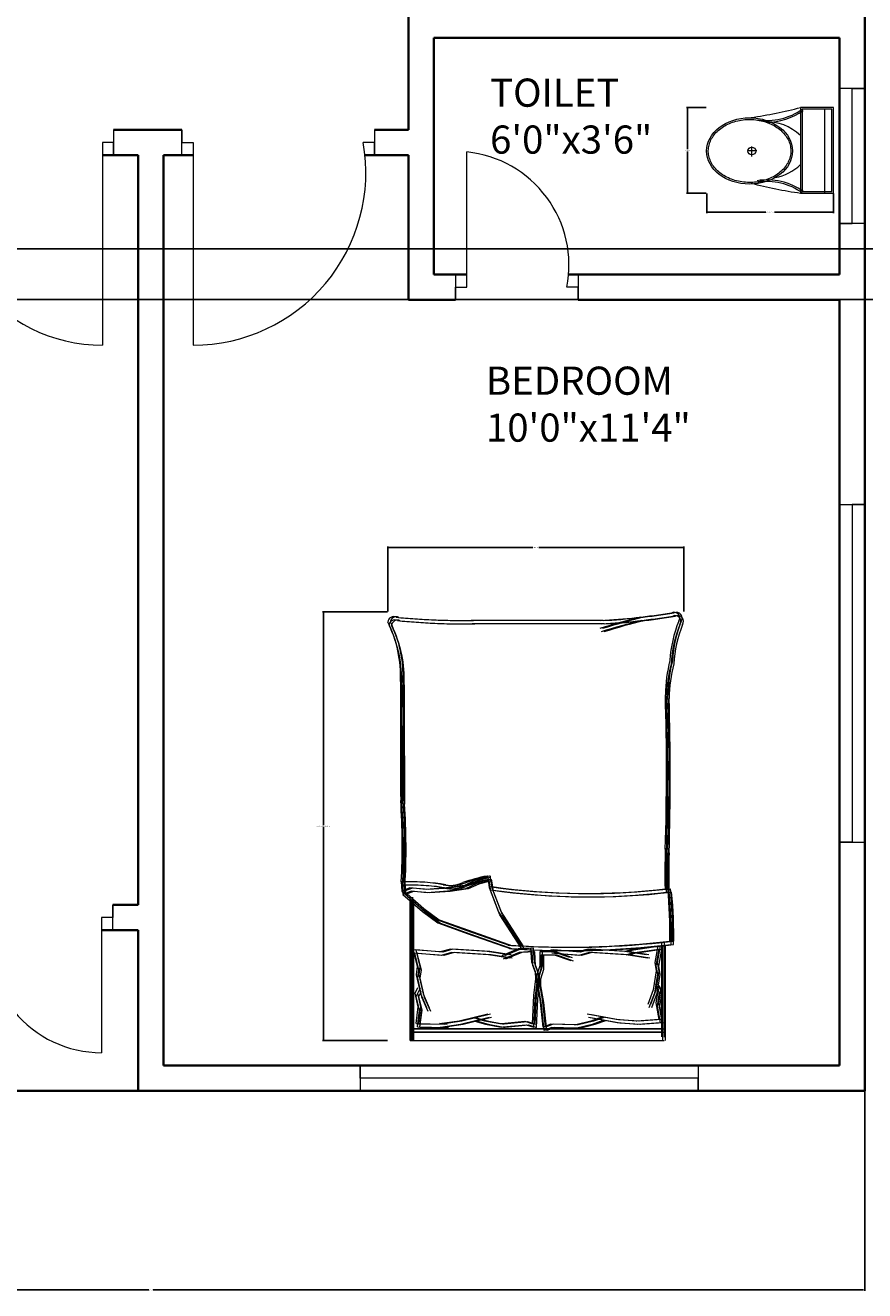
# Model space of a CAD drawing. Units: inches. Extents: x 2234 to 3001, y 1541 to 2386.
# Tile 3 of 12: x 2739 to 2888, y 1667 to 1891. Entities that reach past the tile are written whole.
import ezdxf

# ---------------------------------------------------------------- set-up
doc = ezdxf.new("R2010")
doc.units = ezdxf.units.IN
for name, color, linetype, lineweight in [('A-ANNO-DIMS', 2, 'Continuous', 18), ('A-AREA-IDEN', 7, 'Continuous', 18), ('A-DOOR', 3, 'Continuous', 18), ('A-FLOR-FIXT', 9, 'Continuous', 18), ('A-FURN', 9, 'Continuous', 13), ('A-GLAZ', 4, 'Continuous', 18), ('A-WALL', 7, 'Continuous', 35)]:
    doc.layers.add(name, color=color, linetype=linetype, lineweight=lineweight)
doc.styles.get("Standard").update_dxf_attribs({"font": 'arial.ttf'})
doc.dimstyles.get("Standard").update_dxf_attribs({"dimtxt": 0.18, "dimasz": 0.18, "dimexe": 0.18, "dimexo": 0.0625, "dimgap": 0.09, "dimtad": 0, "dimtih": 1, "dimtoh": 1, "dimdec": 4, "dimzin": 0, "dimdsep": 46, "dimtxsty": 'Standard', "dimcen": 0.09, "dimadec": 0, "dimazin": 0, "dimtfac": 1, "dimtdec": 4, "dimtofl": 0, "dimtmove": 0, "dimatfit": 3, "dimfxl": 1, "dimtolj": 1, "dimtzin": 0, "dimarcsym": 0})

# ---------------------------------------------------------------- blocks, each defined once
blk = doc.blocks.new('A$C31115884')
for p, q in [((283.1, 497.7), (223.4, 497.7)), ((257.5, 466.4), (257.5, 523.2)), ((0, 200), (0, 0)), ((520, 200), (0, 200)), ((10, 190), (10, 10)), ((510, 190), (10, 190)), ((510, 10), (510, 190)), ((520, 0), (520, 200)), ((510, 54.5), (0, 54.5)), ((10, 10), (510, 10)), ((0, 0), (520, 0))]:
    blk.add_line(p, q)
blk.add_circle((255.6, 496.4), 23.6)
for centre, radius, start, end in [((2777.7, -204.6), 2807, 165.4549, 171.71327), ((-294.5, 403.3), 364.7, 324.20913, 9.34987), ((-294.5, 403.3), 374.7, 324.20913, 9.34987), ((805.8, 403.3), 364.7, 170.65013, 215.79087), ((3237, 905), 2807, 188.28673, 194.5451), ((139.5, 406.2), 293.5, 315.84364, 2.65635), ((805.8, 403.3), 374.7, 179.20365, 215.79087), ((383.6, 406.2), 293.5, 190.27735, 224.15636)]:
    blk.add_arc(centre, radius, start, end)
blk.add_ellipse((256.2, 509.9), major_axis=(0, -260.7), ratio=0.772727)
blk.add_open_spline([(256.2, 259.2), (263.1, 259.2), (270, 259.7), (287.8, 262.3), (298.7, 265.1), (319.9, 273.1), (330.2, 278.4), (350.1, 291.1), (359.7, 298.7), (377.7, 315.9), (386.2, 325.5), (401.7, 346.6), (408.8, 358.1), (421.3, 382.5), (426.8, 395.5), (435.9, 422.4), (439.5, 436.4), (444.8, 465.1), (446.5, 479.7), (447.9, 509.2), (447.6, 524), (445, 553.3), (442.7, 567.8), (436.3, 596), (432.1, 609.7), (421.9, 636), (416, 648.6), (402.5, 672.1), (395, 683), (378.6, 703), (369.8, 712.1), (351.1, 728), (341.3, 734.8), (320.9, 746.2), (310.4, 750.7), (288.9, 757.3), (278, 759.4), (256, 761), (245, 760.6), (223.1, 757.2), (212.3, 754.3), (191.1, 746.1), (180.8, 740.7), (160.9, 727.8), (151.4, 720.1), (133.5, 702.7), (125.1, 693), (109.6, 671.7), (102.6, 660.2), (90.2, 635.7), (84.9, 622.7), (76, 595.6), (72.4, 581.6), (67.2, 552.9), (65.6, 538.2), (64.4, 508.8), (64.8, 494), (67.5, 464.7), (69.9, 450.2), (76.6, 422), (80.8, 408.3), (91.1, 382.2), (97.2, 369.7), (110.8, 346.3), (118.4, 335.4), (134.8, 315.6), (143.7, 306.7), (162.4, 290.9), (172.3, 284.2), (192.8, 273), (203.3, 268.6), (224.8, 262.2), (235.8, 260.2), (249.9, 259.3), (253, 259.2), (256.2, 259.2)], degree=3, knots=[0, 0, 0, 0, 0.110105, 0.110105, 0.285049, 0.285049, 0.459994, 0.459994, 0.634938, 0.634938, 0.809882, 0.809882, 0.984827, 0.984827, 1.159771, 1.159771, 1.334715, 1.334715, 1.50966, 1.50966, 1.684604, 1.684604, 1.859549, 1.859549, 2.034493, 2.034493, 2.209437, 2.209437, 2.384382, 2.384382, 2.559326, 2.559326, 2.73427, 2.73427, 2.909215, 2.909215, 3.084159, 3.084159, 3.259103, 3.259103, 3.434048, 3.434048, 3.608992, 3.608992, 3.783936, 3.783936, 3.958881, 3.958881, 4.133825, 4.133825, 4.30877, 4.30877, 4.483714, 4.483714, 4.658658, 4.658658, 4.833603, 4.833603, 5.008547, 5.008547, 5.183491, 5.183491, 5.358436, 5.358436, 5.53338, 5.53338, 5.708324, 5.708324, 5.883269, 5.883269, 6.058213, 6.058213, 6.233158, 6.233158, 6.283185, 6.283185, 6.283185, 6.283185])
blk = doc.blocks.new('WIN-60-A')
for p, q in [((0, 60), (4.5, 60)), ((4.5, 60), (2.25, 60)), ((2.25, 60), (2.25, 0)), ((2.25, 0), (0, 0)), ((0, 0), (4.5, 0))]:
    blk.add_line(p, q)
blk = doc.blocks.new('WIN-24-A')
for p, q in [((0, 24), (4.5, 24)), ((4.5, 24), (2.25, 24)), ((2.25, 24), (2.25, 0)), ((2.25, 0), (0, 0)), ((0, 0), (4.5, 0))]:
    blk.add_line(p, q)
blk = doc.blocks.new('BED-DOUBLE-B')
for p, q in [((37.77, 74.61), (14.78, 74.61)), ((37.77, 74.61), (14.78, 74.61)), ((38.22, 74.59), (15.24, 74.59)), ((38.22, 74.59), (15.24, 74.59)), ((37.98, 74.02), (15, 74.02)), ((37.98, 74.02), (15, 74.02)), ((38.44, 73.99), (15.45, 73.99)), ((38.44, 73.99), (15.46, 73.99)), ((2.39, 28.15), (2.47, 26.53, 3.61)), ((2.39, 28.15), (2.47, 26.53, 3.61)), ((3.9, 27.1), (2.47, 26.53)), ((3.9, 27.1), (2.47, 26.53)), ((2.61, 27.56), (2.68, 25.93, 3.61)), ((2.61, 27.56), (2.68, 25.93, 3.61)), ((2.85, 28.13), (2.92, 26.5, 3.61)), ((2.85, 28.13), (2.93, 26.5, 3.61)), ((4.36, 27.08), (2.92, 26.5)), ((4.36, 27.08), (2.93, 26.5)), ((3.06, 27.54), (3.14, 25.91, 3.61)), ((3.06, 27.54), (3.14, 25.91, 3.61)), ((6.79, 26.81), (3.9, 27.1)), ((6.8, 26.81), (3.9, 27.1)), ((7.25, 26.79), (4.36, 27.08)), ((7.25, 26.79), (4.36, 27.08)), ((10.41, 27.1), (6.79, 26.81)), ((10.41, 27.1), (6.8, 26.81)), ((10.87, 27.08), (7.25, 26.79)), ((10.87, 27.08), (7.25, 26.79)), ((13.59, 27.54), (10.41, 27.1)), ((13.59, 27.54), (10.41, 27.1)), ((14.05, 27.52), (10.87, 27.08)), ((14.05, 27.52), (10.87, 27.08)), ((15.47, 28.4), (13.59, 27.54)), ((15.47, 28.4), (13.59, 27.54)), ((15.68, 27.81), (13.8, 26.94)), ((15.69, 27.81), (13.81, 26.94)), ((15.93, 28.38), (14.05, 27.52)), ((15.93, 28.38), (14.05, 27.52)), ((16.14, 27.79), (14.26, 26.92)), ((16.14, 27.79), (14.26, 26.92)), ((17.79, 28.98), (15.47, 28.4)), ((17.79, 28.98), (15.47, 28.4)), ((18, 28.38), (15.68, 27.81)), ((18, 28.38), (15.69, 27.81)), ((18.24, 28.96), (15.93, 28.38)), ((18.24, 28.96), (15.93, 28.38)), ((18.46, 28.36), (16.14, 27.79)), ((18.46, 28.36), (16.14, 27.79)), ((18.07, 27.1), (17.79, 28.98)), ((18.07, 27.1), (17.79, 28.98)), ((18.29, 26.51), (18, 28.38)), ((18.29, 26.51), (18, 28.38)), ((19.67, 22.91), (18.07, 27.1)), ((19.67, 22.91), (18.07, 27.1)), ((18.53, 27.08), (18.24, 28.96)), ((18.53, 27.08), (18.24, 28.96)), ((18.75, 26.49), (18.46, 28.36)), ((18.75, 26.49), (18.46, 28.36)), ((20.12, 22.89), (18.53, 27.08)), ((20.12, 22.89), (18.53, 27.08)), ((2.47, 26.53), (5.93, 23.49)), ((2.47, 26.53), (5.93, 23.49)), ((4.12, 26.51), (2.68, 25.93)), ((4.12, 26.51), (2.68, 25.93)), ((2.68, 25.93), (6.14, 22.89)), ((2.68, 25.93), (6.14, 22.89)), ((2.92, 26.5), (6.38, 23.47)), ((2.93, 26.5), (6.39, 23.47)), ((4.57, 26.49), (3.14, 25.91)), ((4.57, 26.49), (3.14, 25.91)), ((3.14, 25.91), (6.6, 22.87)), ((3.14, 25.91), (6.6, 22.87)), ((3.96, 0.62), (3.96, 25.46)), ((3.96, 0.62), (3.96, 25.46)), ((7.01, 26.22), (4.12, 26.51)), ((7.01, 26.22), (4.12, 26.51)), ((4.18, 0.02), (4.18, 24.87)), ((4.18, 0.02), (4.18, 24.87)), ((4.42, 0.6), (4.42, 25.44)), ((4.42, 0.6), (4.42, 25.44)), ((7.47, 26.2), (4.57, 26.49)), ((7.47, 26.2), (4.57, 26.49)), ((4.63, 0), (4.63, 24.85)), ((4.63, 0), (4.63, 24.85)), ((10.62, 26.51), (7.01, 26.22)), ((10.62, 26.51), (7.01, 26.22)), ((11.08, 26.49), (7.47, 26.2)), ((11.08, 26.49), (7.47, 26.2)), ((13.8, 26.94), (10.62, 26.51)), ((13.81, 26.94), (10.62, 26.51)), ((14.26, 26.92), (11.08, 26.49)), ((14.26, 26.92), (11.08, 26.49)), ((19.88, 22.32), (18.29, 26.51)), ((19.88, 22.32), (18.29, 26.51)), ((20.34, 22.29), (18.75, 26.49)), ((20.34, 22.29), (18.75, 26.49)), ((5.93, 23.49), (8.67, 21.47)), ((5.93, 23.49), (8.68, 21.47)), ((6.14, 22.89), (8.89, 20.87)), ((6.14, 22.89), (8.89, 20.87)), ((6.38, 23.47), (9.13, 21.45)), ((6.39, 23.47), (9.13, 21.45)), ((6.6, 22.87), (9.35, 20.85)), ((6.6, 22.87), (9.35, 20.85)), ((23.58, 16.85), (19.67, 22.91)), ((23.58, 16.85), (19.67, 22.91)), ((24.04, 16.83), (20.12, 22.89)), ((24.04, 16.83), (20.12, 22.89)), ((8.67, 21.47), (13.88, 19.59)), ((8.68, 21.47), (13.88, 19.59)), ((8.89, 20.87), (14.09, 18.99)), ((8.89, 20.87), (14.09, 18.99)), ((9.13, 21.45), (14.34, 19.57)), ((9.13, 21.45), (14.34, 19.57)), ((9.35, 20.85), (14.55, 18.97)), ((9.35, 20.85), (14.55, 18.97)), ((23.79, 16.25), (19.88, 22.32)), ((23.79, 16.25), (19.88, 22.32)), ((24.25, 16.23), (20.34, 22.29)), ((24.25, 16.23), (20.34, 22.29)), ((13.88, 19.59), (21.67, 16.85)), ((13.88, 19.59), (21.67, 16.85)), ((14.09, 18.99), (21.88, 16.25)), ((14.09, 18.99), (21.88, 16.25)), ((14.34, 19.57), (22.12, 16.83)), ((14.34, 19.57), (22.12, 16.83)), ((14.55, 18.97), (22.34, 16.23)), ((14.55, 18.97), (22.34, 16.23)), ((9.28, 15.72), (4.49, 16.09)), ((4.49, 16.09), (5.22, 13.16)), ((9.29, 15.72), (4.49, 16.09)), ((4.49, 16.09), (5.22, 13.16)), ((9.74, 15.69), (4.95, 16.07)), ((4.95, 16.07), (5.67, 13.14)), ((9.74, 15.69), (4.95, 16.07)), ((4.95, 16.07), (5.67, 13.14)), ((11.12, 16.24), (9.28, 15.72)), ((11.12, 16.24), (9.29, 15.72)), ((11.57, 16.21), (9.74, 15.69)), ((11.57, 16.21), (9.74, 15.69)), ((17.66, 15.83), (11.12, 16.24)), ((17.66, 15.83), (11.12, 16.24)), ((18.12, 15.81), (11.57, 16.21)), ((18.12, 15.81), (11.57, 16.21)), ((21.43, 15.21), (17.66, 15.83)), ((21.43, 15.21), (17.66, 15.83)), ((21.88, 15.19), (18.12, 15.81)), ((21.88, 15.19), (18.12, 15.81)), ((23.12, 16.25), (20.25, 15.05)), ((23.12, 16.25), (20.25, 15.05)), ((23.58, 16.23), (20.71, 15.03)), ((23.58, 16.23), (20.71, 15.03)), ((25.41, 16.39), (23.12, 16.25)), ((25.41, 16.39), (23.12, 16.25)), ((25.62, 15.79), (23.33, 15.65)), ((25.62, 15.79), (23.33, 15.65)), ((25.87, 16.37), (23.58, 16.23)), ((25.87, 16.37), (23.58, 16.23)), ((26.08, 15.77), (23.79, 15.63)), ((26.08, 15.77), (23.79, 15.63)), ((25.57, 13.89), (25.41, 16.39)), ((25.57, 13.89), (25.41, 16.39)), ((25.78, 13.3), (25.62, 15.79)), ((25.78, 13.3), (25.62, 15.79)), ((26.02, 13.87), (25.87, 16.37)), ((26.02, 13.87), (25.87, 16.37)), ((26.24, 13.27), (26.08, 15.77)), ((26.24, 13.27), (26.08, 15.77)), ((27.03, 13.3), (27.03, 15.8)), ((27.03, 15.8), (29.33, 15.8)), ((27.03, 13.3), (27.03, 15.8)), ((27.03, 15.8), (29.33, 15.8)), ((27.49, 13.28), (27.49, 15.78)), ((27.49, 15.78), (29.78, 15.78)), ((27.49, 13.28), (27.49, 15.78)), ((27.49, 15.78), (29.78, 15.78)), ((33.73, 15.72), (28.94, 16.09)), ((33.73, 15.72), (28.94, 16.09)), ((29.33, 15.8), (32.26, 14.78)), ((29.33, 15.8), (32.26, 14.78)), ((34.19, 15.69), (29.4, 16.07)), ((34.19, 15.69), (29.4, 16.07)), ((29.78, 15.78), (32.72, 14.76)), ((29.78, 15.78), (32.72, 14.76)), ((35.56, 16.24), (33.73, 15.72)), ((35.56, 16.24), (33.73, 15.72)), ((36.02, 16.21), (34.19, 15.69)), ((36.02, 16.21), (34.19, 15.69)), ((42.11, 15.83), (35.56, 16.24)), ((42.11, 15.83), (35.56, 16.24)), ((42.57, 15.81), (36.02, 16.21)), ((42.57, 15.81), (36.02, 16.21)), ((42.11, 15.83), (43.17, 16.13)), ((42.11, 15.83), (43.17, 16.13)), ((45.87, 15.21), (42.11, 15.83)), ((45.87, 15.21), (42.11, 15.83)), ((42.57, 15.81), (43.62, 16.11)), ((42.57, 15.81), (43.62, 16.11)), ((46.33, 15.19), (42.57, 15.81)), ((46.33, 15.19), (42.57, 15.81)), ((43.17, 16.13), (47.93, 16.81)), ((43.17, 16.13), (47.93, 16.81)), ((43.38, 15.54), (48.14, 16.21)), ((43.38, 15.54), (48.14, 16.21)), ((43.62, 16.11), (48.38, 16.79)), ((43.62, 16.11), (48.38, 16.79)), ((43.84, 15.52), (48.6, 16.19)), ((43.84, 15.52), (48.6, 16.19)), ((47.93, 16.81), (47.39, 13.84)), ((47.93, 16.81), (47.39, 13.84)), ((48.14, 16.21), (47.6, 13.24)), ((48.14, 16.21), (47.6, 13.24)), ((48.38, 16.79), (47.84, 13.82)), ((48.38, 16.79), (47.84, 13.82)), ((48.6, 16.19), (48.06, 13.22)), ((48.6, 16.19), (48.06, 13.22)), ((48.59, 17.53), (48.59, 0.62)), ((48.59, 17.53), (48.59, 0.62)), ((48.8, 16.93), (48.8, 0.02)), ((48.8, 16.93), (48.8, 0.02)), ((49.05, 17.51), (49.05, 0.6)), ((49.05, 17.51), (49.05, 0.6)), ((49.26, 16.91), (49.26, 0)), ((49.26, 16.91), (49.26, 0)), ((9.5, 15.12), (4.71, 15.5)), ((4.71, 15.5), (5.43, 12.56)), ((9.5, 15.12), (4.71, 15.5)), ((4.71, 15.5), (5.43, 12.56)), ((9.96, 15.1), (5.16, 15.47)), ((5.16, 15.47), (5.89, 12.54)), ((9.96, 15.1), (5.16, 15.47)), ((5.16, 15.47), (5.89, 12.54)), ((11.33, 15.64), (9.5, 15.12)), ((11.33, 15.64), (9.5, 15.12)), ((11.79, 15.62), (9.96, 15.1)), ((11.79, 15.62), (9.96, 15.1)), ((17.87, 15.24), (11.33, 15.64)), ((17.87, 15.24), (11.33, 15.64)), ((18.33, 15.22), (11.79, 15.62)), ((18.33, 15.22), (11.79, 15.62)), ((21.64, 14.61), (17.87, 15.24)), ((21.64, 14.61), (17.87, 15.24)), ((22.1, 14.59), (18.33, 15.22)), ((22.1, 14.59), (18.33, 15.22)), ((23.33, 15.65), (20.47, 14.45)), ((23.33, 15.65), (20.47, 14.45)), ((23.79, 15.63), (20.92, 14.43)), ((23.79, 15.63), (20.92, 14.43)), ((26.21, 12.17), (25.57, 13.89)), ((26.21, 12.17), (25.57, 13.89)), ((26.67, 12.15), (26.02, 13.87)), ((26.67, 12.15), (26.02, 13.87)), ((27.24, 12.7), (27.24, 15.21)), ((27.24, 15.21), (29.54, 15.21)), ((27.24, 12.7), (27.24, 15.21)), ((27.24, 15.21), (29.54, 15.21)), ((27.7, 12.68), (27.7, 15.19)), ((27.7, 15.19), (30, 15.19)), ((27.7, 12.68), (27.7, 15.19)), ((27.7, 15.19), (30, 15.19)), ((33.95, 15.12), (29.15, 15.5)), ((33.95, 15.12), (29.15, 15.5)), ((29.54, 15.21), (32.48, 14.19)), ((29.54, 15.21), (32.48, 14.19)), ((34.4, 15.1), (29.61, 15.47)), ((34.4, 15.1), (29.61, 15.47)), ((30, 15.19), (32.93, 14.17)), ((30, 15.19), (32.93, 14.17)), ((35.78, 15.64), (33.95, 15.12)), ((35.78, 15.64), (33.95, 15.12)), ((36.23, 15.62), (34.4, 15.1)), ((36.23, 15.62), (34.4, 15.1)), ((42.32, 15.24), (35.78, 15.64)), ((42.32, 15.24), (35.78, 15.64)), ((42.78, 15.22), (36.23, 15.62)), ((42.78, 15.22), (36.23, 15.62)), ((42.32, 15.24), (43.38, 15.54)), ((42.32, 15.24), (43.38, 15.54)), ((46.09, 14.61), (42.32, 15.24)), ((46.09, 14.61), (42.32, 15.24)), ((42.78, 15.22), (43.84, 15.52)), ((42.78, 15.22), (43.84, 15.52)), ((46.54, 14.59), (42.78, 15.22)), ((46.54, 14.59), (42.78, 15.22)), ((47.39, 13.84), (47.66, 12.35)), ((47.39, 13.84), (47.66, 12.35)), ((47.84, 13.82), (48.11, 12.33)), ((47.84, 13.82), (48.11, 12.33)), ((5.22, 13.16), (5.04, 11.66)), ((5.22, 13.16), (5.04, 11.66)), ((5.04, 11.66), (5.79, 8.33)), ((5.04, 11.66), (5.79, 8.33)), ((5.43, 12.56), (5.25, 11.07)), ((5.43, 12.56), (5.25, 11.07)), ((5.67, 13.14), (5.5, 11.64)), ((5.67, 13.14), (5.5, 11.64)), ((5.5, 11.64), (6.25, 8.31)), ((5.5, 11.64), (6.25, 8.31)), ((5.89, 12.54), (5.71, 11.04)), ((5.89, 12.54), (5.71, 11.04)), ((26.43, 11.58), (25.78, 13.3)), ((26.43, 11.58), (25.78, 13.3)), ((26.29, 10.96), (26.21, 12.17)), ((26.29, 10.96), (26.21, 12.17)), ((26.88, 11.56), (26.24, 13.27)), ((26.89, 11.56), (26.24, 13.27)), ((26.5, 10.36), (26.43, 11.58)), ((26.5, 10.36), (26.43, 11.58)), ((26.49, 11.54), (27.03, 13.3)), ((26.49, 11.54), (27.03, 13.3)), ((26.49, 10.33), (26.49, 11.54)), ((26.49, 10.33), (26.49, 11.54)), ((26.75, 10.94), (26.67, 12.15)), ((26.75, 10.94), (26.67, 12.15)), ((26.7, 10.95), (27.24, 12.7)), ((26.7, 10.95), (27.24, 12.7)), ((26.96, 10.34), (26.88, 11.56)), ((26.96, 10.34), (26.89, 11.56)), ((26.95, 11.52), (27.49, 13.28)), ((26.95, 11.52), (27.49, 13.28)), ((26.95, 10.31), (26.95, 11.52)), ((26.95, 10.31), (26.95, 11.52)), ((27.16, 10.93), (27.7, 12.68)), ((27.16, 10.93), (27.7, 12.68)), ((47.66, 12.35), (47.12, 8.98)), ((47.66, 12.35), (47.12, 8.98)), ((47.87, 11.76), (47.33, 8.38)), ((47.87, 11.76), (47.33, 8.38)), ((48.11, 12.33), (47.57, 8.96)), ((48.11, 12.33), (47.57, 8.96)), ((47.6, 13.24), (47.87, 11.76)), ((47.6, 13.24), (47.87, 11.76)), ((48.33, 11.74), (47.79, 8.36)), ((48.33, 11.74), (47.79, 8.36)), ((48.06, 13.22), (48.33, 11.74)), ((48.06, 13.22), (48.33, 11.74)), ((4.84, 8.4), (5.32, 9.38)), ((4.84, 8.4), (5.32, 9.38)), ((5.25, 11.07), (6, 7.73)), ((5.25, 11.07), (6, 7.73)), ((5.3, 8.38), (5.78, 9.36)), ((5.3, 8.38), (5.78, 9.36)), ((5.71, 11.04), (6.46, 7.71)), ((5.71, 11.04), (6.46, 7.71)), ((25.94, 7.96), (26.29, 10.96)), ((25.94, 7.96), (26.29, 10.96)), ((26.15, 7.37), (26.5, 10.36)), ((26.15, 7.37), (26.5, 10.36)), ((26.39, 7.94), (26.75, 10.94)), ((26.39, 7.94), (26.75, 10.94)), ((27.03, 7.36), (26.49, 10.33)), ((27.03, 7.36), (26.49, 10.33)), ((26.61, 7.35), (26.96, 10.34)), ((26.61, 7.35), (26.96, 10.34)), ((26.7, 9.73), (26.7, 10.95)), ((26.7, 9.73), (26.7, 10.95)), ((27.24, 6.76), (26.7, 9.73)), ((27.24, 6.76), (26.7, 9.73)), ((27.49, 7.34), (26.95, 10.31)), ((27.49, 7.34), (26.95, 10.31)), ((27.16, 9.71), (27.16, 10.93)), ((27.16, 9.71), (27.16, 10.93)), ((27.7, 6.74), (27.16, 9.71)), ((27.7, 6.74), (27.16, 9.71)), ((48.06, 9.11), (47.52, 10.06)), ((48.06, 9.11), (47.52, 10.06)), ((47.66, 6.68), (48.06, 9.11)), ((47.66, 6.68), (48.06, 9.11)), ((48.27, 8.52), (47.73, 9.46)), ((48.27, 8.52), (47.73, 9.46)), ((48.52, 9.09), (47.98, 10.04)), ((48.52, 9.09), (47.98, 10.04)), ((48.11, 6.66), (48.52, 9.09)), ((48.11, 6.66), (48.52, 9.09)), ((48.73, 8.5), (48.19, 9.44)), ((48.73, 8.5), (48.19, 9.44)), ((5.39, 6), (4.84, 8.4)), ((5.39, 6), (4.84, 8.4)), ((5.05, 7.81), (5.53, 8.78)), ((5.05, 7.81), (5.53, 8.78)), ((5.61, 5.41), (5.05, 7.81)), ((5.61, 5.41), (5.05, 7.81)), ((5.85, 5.98), (5.3, 8.38)), ((5.85, 5.98), (5.3, 8.38)), ((5.51, 7.79), (5.99, 8.76)), ((5.51, 7.79), (5.99, 8.76)), ((6.06, 5.39), (5.51, 7.79)), ((6.07, 5.39), (5.51, 7.79)), ((5.79, 8.33), (6.89, 5.83)), ((5.79, 8.33), (6.89, 5.83)), ((6, 7.73), (7.11, 5.23)), ((6, 7.73), (7.11, 5.23)), ((6.25, 8.31), (7.35, 5.81)), ((6.25, 8.31), (7.35, 5.81)), ((6.46, 7.71), (7.56, 5.21)), ((6.46, 7.71), (7.56, 5.21)), ((25.71, 2.94), (25.94, 7.96)), ((25.71, 2.94), (25.94, 7.96)), ((25.92, 2.35), (26.15, 7.37)), ((25.92, 2.35), (26.15, 7.37)), ((26.17, 2.92), (26.39, 7.94)), ((26.17, 2.92), (26.39, 7.94)), ((26.38, 2.33), (26.61, 7.35)), ((26.38, 2.33), (26.61, 7.35)), ((27.57, 2.36), (27.03, 7.36)), ((27.57, 2.36), (27.03, 7.36)), ((27.78, 1.77), (27.24, 6.76)), ((27.78, 1.77), (27.24, 6.76)), ((28.03, 2.34), (27.49, 7.34)), ((28.03, 2.34), (27.49, 7.34)), ((47.12, 8.98), (46.17, 6.41)), ((47.12, 8.98), (46.17, 6.41)), ((47.33, 8.38), (46.38, 5.82)), ((47.33, 8.38), (46.38, 5.82)), ((47.57, 8.96), (46.63, 6.39)), ((47.57, 8.96), (46.63, 6.39)), ((47.79, 8.36), (46.84, 5.8)), ((47.79, 8.36), (46.84, 5.8)), ((47.87, 6.09), (48.27, 8.52)), ((47.87, 6.09), (48.27, 8.52)), ((48.33, 6.07), (48.73, 8.5)), ((48.33, 6.07), (48.73, 8.5)), ((5.04, 3.01), (5.39, 6)), ((5.04, 3.01), (5.39, 6)), ((5.25, 2.41), (5.61, 5.41)), ((5.25, 2.41), (5.61, 5.41)), ((5.5, 2.98), (5.85, 5.98)), ((5.5, 2.98), (5.85, 5.98)), ((5.71, 2.39), (6.06, 5.39)), ((5.71, 2.39), (6.07, 5.39)), ((12.69, 3.48), (17.76, 4.75)), ((12.7, 3.48), (17.76, 4.75)), ((13.15, 3.46), (18.21, 4.73)), ((13.15, 3.46), (18.21, 4.73)), ((28.24, 1.75), (27.7, 6.74)), ((28.24, 1.75), (27.7, 6.74)), ((40.53, 3.71), (35.4, 4.66)), ((40.53, 3.71), (35.4, 4.66)), ((40.98, 3.69), (35.85, 4.64)), ((40.98, 3.69), (35.85, 4.64)), ((48.2, 3.71), (47.66, 6.68)), ((48.2, 3.71), (47.66, 6.68)), ((48.41, 3.12), (47.87, 6.09)), ((48.41, 3.12), (47.87, 6.09)), ((48.65, 3.69), (48.11, 6.66)), ((48.65, 3.69), (48.11, 6.66)), ((48.87, 3.1), (48.33, 6.07)), ((48.87, 3.1), (48.33, 6.07)), ((5.04, 3.01), (10.08, 2.91)), ((5.04, 3.01), (10.09, 2.91)), ((5.25, 2.41), (10.3, 2.32)), ((5.25, 2.41), (10.3, 2.32)), ((5.5, 2.98), (10.54, 2.89)), ((5.5, 2.98), (10.54, 2.89)), ((5.71, 2.39), (10.76, 2.3)), ((5.71, 2.39), (10.76, 2.3)), ((9.15, 2.99), (12.69, 3.48)), ((9.15, 2.99), (12.7, 3.48)), ((10.08, 2.91), (9.15, 2.99)), ((10.09, 2.91), (9.15, 2.99)), ((9.36, 2.39), (12.91, 2.89)), ((9.36, 2.39), (12.91, 2.89)), ((10.3, 2.32), (9.36, 2.39)), ((10.3, 2.32), (9.36, 2.39)), ((9.61, 2.97), (13.15, 3.46)), ((9.61, 2.97), (13.15, 3.46)), ((10.54, 2.89), (9.61, 2.97)), ((10.54, 2.89), (9.61, 2.97)), ((9.82, 2.37), (13.37, 2.87)), ((9.82, 2.37), (13.37, 2.87)), ((10.76, 2.3), (9.82, 2.37)), ((10.76, 2.3), (9.82, 2.37)), ((12.91, 2.89), (17.97, 4.15)), ((12.91, 2.89), (17.97, 4.15)), ((13.37, 2.87), (18.43, 4.13)), ((13.37, 2.87), (18.43, 4.13)), ((15.23, 4.05), (17.16, 3.49)), ((15.23, 4.05), (17.16, 3.49)), ((15.44, 3.45), (17.37, 2.89)), ((15.44, 3.45), (17.37, 2.89)), ((15.69, 4.03), (17.61, 3.47)), ((15.69, 4.03), (17.62, 3.47)), ((15.9, 3.43), (17.83, 2.87)), ((15.9, 3.43), (17.83, 2.87)), ((17.16, 3.49), (19.89, 2.99)), ((17.16, 3.49), (19.89, 2.99)), ((17.37, 2.89), (20.11, 2.39)), ((17.37, 2.89), (20.11, 2.39)), ((17.61, 3.47), (20.35, 2.97)), ((17.62, 3.47), (20.35, 2.97)), ((17.83, 2.87), (20.56, 2.37)), ((17.83, 2.87), (20.56, 2.37)), ((19.89, 2.99), (20.19, 3.01)), ((19.89, 2.99), (20.19, 3.01)), ((20.11, 2.39), (20.41, 2.41)), ((20.11, 2.39), (20.41, 2.41)), ((20.19, 3.01), (24.33, 3.4)), ((20.19, 3.01), (24.33, 3.4)), ((20.35, 2.97), (20.65, 2.98)), ((20.35, 2.97), (20.65, 2.98)), ((20.41, 2.41), (24.54, 2.8)), ((20.41, 2.41), (24.54, 2.8)), ((20.56, 2.37), (20.86, 2.39)), ((20.56, 2.37), (20.86, 2.39)), ((20.65, 2.98), (24.79, 3.38)), ((20.65, 2.98), (24.79, 3.38)), ((20.86, 2.39), (25, 2.78)), ((20.86, 2.39), (25, 2.78)), ((24.33, 3.4), (25.71, 2.94)), ((24.33, 3.4), (25.71, 2.94)), ((24.54, 2.8), (25.92, 2.35)), ((24.54, 2.8), (25.92, 2.35)), ((24.79, 3.38), (26.17, 2.92)), ((24.79, 3.38), (26.17, 2.92)), ((25, 2.78), (26.38, 2.33)), ((25, 2.78), (26.38, 2.33)), ((28.92, 2.9), (27.57, 2.36)), ((28.92, 2.9), (27.57, 2.36)), ((29.13, 2.31), (27.78, 1.77)), ((29.13, 2.31), (27.78, 1.77)), ((29.38, 2.88), (28.03, 2.34)), ((29.38, 2.88), (28.03, 2.34)), ((29.59, 2.29), (28.24, 1.75)), ((29.59, 2.29), (28.24, 1.75)), ((33.07, 2.77), (28.92, 2.9)), ((33.07, 2.77), (28.92, 2.9)), ((33.29, 2.17), (29.13, 2.31)), ((33.29, 2.17), (29.13, 2.31)), ((33.53, 2.75), (29.38, 2.88)), ((33.53, 2.75), (29.38, 2.88)), ((33.74, 2.15), (29.59, 2.29)), ((33.74, 2.15), (29.59, 2.29)), ((33.37, 2.77), (33.07, 2.77)), ((33.37, 2.77), (33.07, 2.77)), ((36.07, 3.44), (33.37, 2.77)), ((36.07, 3.44), (33.37, 2.77)), ((33.83, 2.75), (33.53, 2.75)), ((33.83, 2.75), (33.53, 2.75)), ((36.29, 2.85), (33.59, 2.17)), ((36.29, 2.85), (33.59, 2.17)), ((36.53, 3.42), (33.83, 2.75)), ((36.53, 3.42), (33.83, 2.75)), ((36.74, 2.83), (34.04, 2.15)), ((36.74, 2.83), (34.04, 2.15)), ((40.74, 3.12), (35.61, 4.06)), ((40.74, 3.12), (35.61, 4.06)), ((37.96, 4.12), (36.07, 3.44)), ((37.96, 4.12), (36.07, 3.44)), ((41.2, 3.1), (36.07, 4.04)), ((41.2, 3.1), (36.07, 4.04)), ((38.17, 3.52), (36.29, 2.85)), ((38.18, 3.52), (36.29, 2.85)), ((38.42, 4.1), (36.53, 3.42)), ((38.42, 4.1), (36.53, 3.42)), ((38.63, 3.5), (36.74, 2.83)), ((38.63, 3.5), (36.74, 2.83)), ((44.1, 3.44), (40.53, 3.71)), ((44.1, 3.44), (40.53, 3.71)), ((44.31, 2.85), (40.74, 3.12)), ((44.31, 2.85), (40.74, 3.12)), ((44.55, 3.42), (40.98, 3.69)), ((44.55, 3.42), (40.98, 3.69)), ((44.77, 2.83), (41.2, 3.1)), ((44.77, 2.83), (41.2, 3.1)), ((44.19, 3.43), (44.1, 3.44)), ((44.2, 3.43), (44.1, 3.44)), ((48.19, 3.73), (44.19, 3.43)), ((48.19, 3.73), (44.2, 3.43)), ((44.41, 2.83), (44.31, 2.85)), ((44.41, 2.83), (44.31, 2.85)), ((48.41, 3.14), (44.41, 2.83)), ((48.41, 3.14), (44.41, 2.83)), ((44.65, 3.41), (44.55, 3.42)), ((44.65, 3.41), (44.55, 3.42)), ((48.65, 3.71), (44.65, 3.41)), ((48.65, 3.71), (44.65, 3.41)), ((44.87, 2.81), (44.77, 2.83)), ((44.87, 2.81), (44.77, 2.83)), ((48.86, 3.12), (44.87, 2.81)), ((48.86, 3.12), (44.87, 2.81)), ((48.59, 2.05), (3.96, 2.05)), ((48.59, 2.05), (3.96, 2.05)), ((3.96, 0.02), (3.96, 0.62)), ((3.96, 0.02), (48.59, 0.02)), ((48.8, 1.45), (4.18, 1.45)), ((48.8, 1.45), (4.18, 1.45)), ((49.05, 2.03), (4.42, 2.03)), ((49.05, 2.03), (4.42, 2.03)), ((4.42, 0), (4.42, 0.6)), ((49.26, 1.43), (4.63, 1.43)), ((49.26, 1.43), (4.63, 1.43)), ((33.59, 2.17), (33.29, 2.17)), ((33.59, 2.17), (33.29, 2.17)), ((34.04, 2.15), (33.74, 2.15)), ((34.04, 2.15), (33.74, 2.15)), ((4.42, 0), (49.05, 0))]:
    blk.add_line(p, q)
for centre, radius, start, end in [((1.03, 74.26), 1.03, 62.6588, 176.02), ((1.03, 74.26), 1.03, 62.6588, 176.02), ((-19.28, 64.73), 21.54, 357.4714, 26.4681), ((-19.28, 64.73), 21.54, 357.4714, 26.4681), ((1.24, 73.67), 1.03, 62.6588, 176.02), ((1.24, 73.67), 1.03, 62.6588, 176.02), ((1.48, 74.24), 1.03, 62.6588, 176.02), ((1.49, 74.24), 1.03, 62.6588, 176.02), ((-18.82, 64.71), 21.54, 357.4714, 26.4681), ((-18.82, 64.71), 21.54, 357.4714, 26.4681), ((1.7, 73.64), 1.03, 62.6588, 176.02), ((1.7, 73.64), 1.03, 62.6588, 176.02), ((13.41, 198.83), 124.23, 264.4998, 270.6351), ((13.41, 198.83), 124.23, 264.4998, 270.6351), ((13.62, 198.23), 124.23, 264.4998, 270.6351), ((13.62, 198.23), 124.23, 264.4998, 270.6351), ((13.86, 198.81), 124.23, 264.4998, 270.6351), ((13.86, 198.81), 124.23, 264.4998, 270.6351), ((14.08, 198.21), 124.23, 264.4998, 270.6351), ((14.08, 198.21), 124.23, 264.4998, 270.6351), ((67.91, -21.52), 99.41, 103.3832, 107.7053), ((67.91, -21.52), 99.41, 103.3832, 107.7053), ((31.83, 188.15), 113.69, 272.9958, 279.4091), ((31.83, 188.15), 113.69, 272.9958, 279.4091), ((68.13, -22.12), 99.41, 103.3832, 107.7053), ((68.13, -22.12), 99.41, 103.3832, 107.7053), ((32.04, 187.55), 113.69, 272.9958, 279.4091), ((32.04, 187.55), 113.69, 272.9958, 279.4091), ((68.37, -21.54), 99.41, 103.3832, 107.7053), ((68.37, -21.54), 99.41, 103.3832, 107.7053), ((32.28, 188.13), 113.69, 272.9958, 279.4091), ((32.28, 188.13), 113.69, 272.9958, 279.4091), ((68.58, -22.14), 99.41, 103.3832, 107.7053), ((68.58, -22.14), 99.41, 103.3832, 107.7053), ((32.5, 187.53), 113.69, 272.9958, 279.4091), ((32.5, 187.53), 113.69, 272.9958, 279.4091), ((72.06, 66.24), 22, 157.9751, 176.652), ((72.06, 66.24), 22, 157.9751, 176.652), ((50.82, 75.05), 1.02, 326.1736, 113.4781), ((50.82, 75.05), 1.02, 326.1736, 113.4781), ((72.51, 66.22), 22, 157.9751, 176.652), ((72.51, 66.22), 22, 157.9751, 176.652), ((51.03, 74.46), 1.02, 326.1736, 113.4781), ((51.03, 74.46), 1.02, 326.1736, 113.4781), ((51.27, 75.03), 1.02, 326.1736, 113.4781), ((51.27, 75.03), 1.02, 326.1736, 113.4781), ((51.49, 74.44), 1.02, 326.1736, 113.4781), ((51.49, 74.44), 1.02, 326.1736, 113.4781), ((-19.07, 64.14), 21.54, 357.4714, 26.4681), ((-19.07, 64.14), 21.54, 357.4714, 26.4681), ((-18.61, 64.12), 21.54, 357.4714, 26.4681), ((-18.61, 64.12), 21.54, 357.4714, 26.4681), ((72.27, 65.64), 22, 157.9751, 176.652), ((72.27, 65.64), 22, 157.9751, 176.652), ((72.73, 65.62), 22, 157.9751, 176.652), ((72.73, 65.62), 22, 157.9751, 176.652), ((76.95, 60.86), 27.67, 166.0648, 178.9113), ((76.95, 60.86), 27.67, 166.0648, 178.9113), ((77.41, 60.84), 27.67, 166.0648, 178.9113), ((77.41, 60.84), 27.67, 166.0648, 178.9113), ((77.16, 60.26), 27.67, 166.0648, 178.9113), ((77.16, 60.26), 27.67, 166.0648, 178.9113), ((77.62, 60.24), 27.67, 166.0648, 178.9113), ((77.62, 60.24), 27.67, 166.0648, 178.9113), ((4261.85, 63.95), 4259.62, 180.00217, 180.28689), ((4261.85, 63.95), 4259.62, 180.00217, 180.28689), ((4262.07, 63.35), 4259.62, 180.00217, 180.28689), ((4262.07, 63.35), 4259.62, 180.00217, 180.28689), ((4262.31, 63.92), 4259.62, 180.00217, 180.28689), ((4262.31, 63.92), 4259.62, 180.00217, 180.28689), ((4262.53, 63.33), 4259.62, 180.00217, 180.28689), ((4262.53, 63.33), 4259.62, 180.00217, 180.28689), ((-400.87, 47.88), 450.36, 358.2277, 1.7185), ((-400.87, 47.88), 450.36, 358.2277, 1.7185), ((-400.66, 47.28), 450.36, 358.2277, 1.7185), ((-400.66, 47.28), 450.36, 358.2277, 1.7185), ((-400.41, 47.86), 450.36, 358.2277, 1.7185), ((-400.41, 47.86), 450.36, 358.2277, 1.7185), ((-400.2, 47.26), 450.36, 358.2277, 1.7185), ((-400.2, 47.26), 450.36, 358.2277, 1.7185), ((-118.36, 34.53), 120.92, 356.9791, 3.8365), ((-118.36, 34.53), 120.92, 356.9791, 3.8365), ((-118.14, 33.93), 120.92, 356.9791, 3.8365), ((-118.14, 33.93), 120.92, 356.9791, 3.8365), ((-117.9, 34.51), 120.92, 356.9791, 3.8365), ((-117.9, 34.51), 120.92, 356.9791, 3.8365), ((-117.69, 33.91), 120.92, 356.9791, 3.8365), ((-117.69, 33.91), 120.92, 356.9791, 3.8365), ((208.05, 29.73), 158.84, 178.4762, 181.0082), ((208.06, 29.73), 158.84, 178.4762, 181.0082), ((208.51, 29.7), 158.84, 178.4762, 181.0082), ((208.51, 29.7), 158.84, 178.4762, 181.0082), ((208.27, 29.13), 158.84, 178.4762, 181.0082), ((208.27, 29.13), 158.84, 178.4762, 181.0082), ((208.73, 29.11), 158.84, 178.4762, 181.0082), ((208.73, 29.11), 158.84, 178.4762, 181.0082), ((3.91, -5.6), 33.79, 79.8763, 92.5657), ((3.91, -5.6), 33.79, 79.8763, 92.5657), ((4.12, -6.19), 33.79, 79.8763, 92.5657), ((4.12, -6.19), 33.79, 79.8763, 92.5657), ((4.36, -5.62), 33.79, 79.8763, 92.5657), ((4.36, -5.62), 33.79, 79.8763, 92.5657), ((4.58, -6.22), 33.79, 79.8763, 92.5657), ((4.58, -6.22), 33.79, 79.8763, 92.5657), ((10.99, 33.36), 5.81, 258.6608, 293.7384), ((10.99, 33.36), 5.81, 258.6608, 293.7384), ((11.2, 32.76), 5.81, 258.6608, 293.7384), ((11.2, 32.76), 5.81, 258.6608, 293.7384), ((11.44, 33.34), 5.81, 258.6608, 293.7384), ((11.44, 33.34), 5.81, 258.6608, 293.7384), ((11.66, 32.74), 5.81, 258.6608, 293.7384), ((11.66, 32.74), 5.81, 258.6608, 293.7384), ((22.74, 2), 27.69, 100.6617, 109.8806), ((22.74, 2), 27.69, 100.6617, 109.8806), ((22.96, 1.4), 27.69, 100.6617, 109.8806), ((22.96, 1.4), 27.69, 100.6617, 109.8806), ((23.2, 1.98), 27.69, 100.6617, 109.8806), ((23.2, 1.98), 27.69, 100.6617, 109.8806), ((23.41, 1.38), 27.69, 100.6617, 109.8806), ((23.41, 1.38), 27.69, 100.6617, 109.8806), ((17.62, 29.04), 0.172, 340.2464, 91.1377), ((17.62, 29.04), 0.172, 340.2464, 91.1377), ((17.84, 28.44), 0.172, 340.2464, 91.1377), ((17.84, 28.44), 0.172, 340.2464, 91.1377), ((35.25, 146.58), 120.47, 261.7845, 276.9006), ((35.25, 146.58), 120.47, 261.7845, 276.9006), ((18.08, 29.02), 0.172, 340.2464, 91.1377), ((18.08, 29.02), 0.172, 340.2464, 91.1377), ((18.29, 28.42), 0.172, 340.2464, 91.1377), ((18.29, 28.42), 0.172, 340.2464, 91.1377), ((35.71, 146.56), 120.47, 261.7845, 276.9006), ((35.71, 146.56), 120.47, 261.7845, 276.9006), ((-27.69, 19.38), 77.79, 358.7218, 5.604), ((-27.69, 19.38), 77.79, 358.7218, 5.604), ((35.47, 145.98), 120.47, 261.7845, 276.9006), ((35.47, 145.98), 120.47, 261.7845, 276.9006), ((35.92, 145.96), 120.47, 261.7845, 276.9006), ((35.92, 145.96), 120.47, 261.7845, 276.9006), ((-27.47, 18.79), 77.79, 358.7218, 5.604), ((-27.47, 18.79), 77.79, 358.7218, 5.604), ((-27.23, 19.36), 77.79, 358.7218, 5.604), ((-27.23, 19.36), 77.79, 358.7218, 5.604), ((-27.02, 18.76), 77.79, 358.7218, 5.604), ((-27.02, 18.76), 77.79, 358.7218, 5.604), ((31.89, 170.61), 154.04, 266.0865, 276.7821), ((31.89, 170.61), 154.04, 266.0865, 276.7821), ((32.1, 170.01), 154.04, 266.0865, 276.7821), ((32.1, 170.01), 154.04, 266.0865, 276.7821), ((32.35, 170.59), 154.04, 266.0865, 276.7821), ((32.35, 170.59), 154.04, 266.0865, 276.7821), ((32.56, 169.99), 154.04, 266.0865, 276.7821), ((32.56, 169.99), 154.04, 266.0865, 276.7821)]:
    blk.add_arc(centre, radius, start, end)
blk = doc.blocks.new('*D23')
at = {"layer": 'A-ANNO-DIMS', "color": 0, "lineweight": -2, "transparency": 16777216}
for p, q in [((2860.19, 1861.49), (2860.19, 1857.99)), ((2882.73, 1861.49), (2882.73, 1857.99)), ((2860.37, 1858.17), (2870.68, 1858.17)), ((2882.55, 1858.17), (2872.23, 1858.17))]:
    blk.add_line(p, q, dxfattribs=at)
at = {"layer": 'A-ANNO-DIMS', "color": 0, "transparency": 16777216}
for points in [[(2860.37, 1858.2), (2860.37, 1858.14), (2860.19, 1858.17)], [(2882.55, 1858.2), (2882.55, 1858.14), (2882.73, 1858.17)]]:
    blk.add_solid(points, dxfattribs=at)
at = {"layer": 'Defpoints', "color": 0, "transparency": 16777216}
for p in [(2860.19, 1861.55), (2882.73, 1861.55), (2860.19, 1858.17)]:
    blk.add_point(p, dxfattribs=at)
at = {"layer": 'A-ANNO-DIMS', "color": 0, "transparency": 16777216, "insert": (2871.46, 1858.17), "char_height": 0.18, "attachment_point": 5}
blk.add_mtext('\\A1;WC 23 TYP.', dxfattribs=at)
blk = doc.blocks.new('*D24')
at = {"layer": 'A-ANNO-DIMS', "color": 0, "lineweight": -2, "transparency": 16777216}
for p, q in [((2860.13, 1876.76), (2856.63, 1876.76)), ((2856.81, 1876.58), (2856.81, 1869.33)), ((2856.81, 1861.73), (2856.81, 1868.97)), ((2860.13, 1861.55), (2856.63, 1861.55))]:
    blk.add_line(p, q, dxfattribs=at)
at = {"layer": 'A-ANNO-DIMS', "color": 0, "transparency": 16777216}
for points in [[(2856.78, 1876.58), (2856.84, 1876.58), (2856.81, 1876.76)], [(2856.78, 1861.73), (2856.84, 1861.73), (2856.81, 1861.55)]]:
    blk.add_solid(points, dxfattribs=at)
at = {"layer": 'Defpoints', "color": 0, "transparency": 16777216}
for p in [(2856.81, 1876.76), (2860.19, 1876.76), (2860.19, 1861.55)]:
    blk.add_point(p, dxfattribs=at)
at = {"layer": 'A-ANNO-DIMS', "color": 0, "transparency": 16777216, "insert": (2856.81, 1869.15), "char_height": 0.18, "attachment_point": 5}
blk.add_mtext('\\A1;15 TYP.', dxfattribs=at)
blk = doc.blocks.new('*D37')
at = {"layer": 'A-ANNO-DIMS', "color": 0, "lineweight": -2, "transparency": 16777216}
for p, q in [((2803.5, 1787.2), (2791.96, 1787.2)), ((2792.14, 1787.02), (2792.14, 1749.3)), ((2792.14, 1711.21), (2792.14, 1748.93)), ((2803.5, 1711.03), (2791.96, 1711.03))]:
    blk.add_line(p, q, dxfattribs=at)
at = {"layer": 'A-ANNO-DIMS', "color": 0, "transparency": 16777216}
for points in [[(2792.11, 1787.02), (2792.17, 1787.02), (2792.14, 1787.2)], [(2792.11, 1711.21), (2792.17, 1711.21), (2792.14, 1711.03)]]:
    blk.add_solid(points, dxfattribs=at)
at = {"layer": 'Defpoints', "color": 0, "transparency": 16777216}
for p in [(2792.14, 1787.2), (2803.57, 1787.2), (2803.57, 1711.03)]:
    blk.add_point(p, dxfattribs=at)
at = {"layer": 'A-ANNO-DIMS', "color": 0, "transparency": 16777216, "insert": (2792.14, 1749.11), "char_height": 0.18, "attachment_point": 5}
blk.add_mtext('\\A1;DOUBLE BED B 76 TYP.', dxfattribs=at)
blk = doc.blocks.new('*D38')
at = {"layer": 'A-ANNO-DIMS', "color": 0, "lineweight": -2, "transparency": 16777216}
for p, q in [((2803.57, 1787.26), (2803.57, 1798.8)), ((2803.75, 1798.62), (2829.33, 1798.62)), ((2855.97, 1798.62), (2830.39, 1798.62)), ((2856.15, 1787.26), (2856.15, 1798.8))]:
    blk.add_line(p, q, dxfattribs=at)
at = {"layer": 'A-ANNO-DIMS', "color": 0, "transparency": 16777216}
for points in [[(2803.75, 1798.65), (2803.75, 1798.59), (2803.57, 1798.62)], [(2855.97, 1798.65), (2855.97, 1798.59), (2856.15, 1798.62)]]:
    blk.add_solid(points, dxfattribs=at)
at = {"layer": 'Defpoints', "color": 0, "transparency": 16777216}
for p in [(2856.15, 1798.62), (2803.57, 1787.2), (2856.15, 1787.2)]:
    blk.add_point(p, dxfattribs=at)
at = {"layer": 'A-ANNO-DIMS', "color": 0, "transparency": 16777216, "insert": (2829.86, 1798.62), "char_height": 0.18, "attachment_point": 5}
blk.add_mtext('\\A1;53 TYP.', dxfattribs=at)
blk = doc.blocks.new('*D66')
at = {"layer": 'A-ANNO-DIMS', "color": 0, "lineweight": -2, "transparency": 16777216}
for p, q in [((2634.82, 1851.65), (2923.78, 1851.65)), ((2923.6, 1851.47), (2923.6, 1847.33)), ((2923.6, 1842.83), (2923.6, 1846.97)), ((2639.32, 1842.65), (2923.78, 1842.65))]:
    blk.add_line(p, q, dxfattribs=at)
at = {"layer": 'A-ANNO-DIMS', "color": 0, "transparency": 16777216}
for points in [[(2923.57, 1851.47), (2923.63, 1851.47), (2923.6, 1851.65)], [(2923.57, 1842.83), (2923.63, 1842.83), (2923.6, 1842.65)]]:
    blk.add_solid(points, dxfattribs=at)
at = {"layer": 'Defpoints', "color": 0, "transparency": 16777216}
for p in [(2634.75, 1851.65), (2923.6, 1851.65), (2639.25, 1842.65)]:
    blk.add_point(p, dxfattribs=at)
at = {"layer": 'A-ANNO-DIMS', "color": 0, "transparency": 16777216, "insert": (2923.6, 1847.15), "char_height": 0.18, "attachment_point": 5}
blk.add_mtext('\\A1;9', dxfattribs=at)
blk = doc.blocks.new('*D74')
at = {"layer": 'A-ANNO-DIMS', "color": 0, "lineweight": -2, "transparency": 16777216}
for p, q in [((2634.75, 1706.55), (2634.75, 1666.58)), ((2888.25, 1702.05), (2888.25, 1666.58)), ((2634.93, 1666.76), (2761.11, 1666.76)), ((2888.07, 1666.76), (2761.9, 1666.76))]:
    blk.add_line(p, q, dxfattribs=at)
at = {"layer": 'A-ANNO-DIMS', "color": 0, "transparency": 16777216}
for points in [[(2634.93, 1666.79), (2634.93, 1666.73), (2634.75, 1666.76)], [(2888.07, 1666.79), (2888.07, 1666.73), (2888.25, 1666.76)]]:
    blk.add_solid(points, dxfattribs=at)
at = {"layer": 'Defpoints', "color": 0, "transparency": 16777216}
for p in [(2634.75, 1706.61), (2888.25, 1702.11), (2888.25, 1666.76)]:
    blk.add_point(p, dxfattribs=at)
at = {"layer": 'A-ANNO-DIMS', "color": 0, "transparency": 16777216, "insert": (2761.5, 1666.76), "char_height": 0.18, "attachment_point": 5}
blk.add_mtext('\\A1;253.5', dxfattribs=at)

msp = doc.modelspace()

# ---------------------------------------------------------------- linework, layer by layer
at = {"layer": 'A-DOOR'}
for p, q in [((2754.867, 1872.7928), (2754.867, 1868.2928)), ((2766.9897, 1868.2928), (2766.9897, 1872.7928)), ((2766.9897, 1872.7928), (2766.9897, 1870.5428)), ((2801.2028, 1872.7928), (2801.2028, 1868.2928)), ((2754.867, 1870.5428), (2752.867, 1870.5428)), ((2752.867, 1870.5428), (2752.867, 1834.5428)), ((2754.867, 1868.2928), (2754.867, 1870.5428)), ((2766.9897, 1870.5428), (2768.9897, 1870.5428)), ((2768.9897, 1870.5428), (2768.9897, 1834.5428)), ((2801.2028, 1870.5428), (2799.2028, 1870.5428)), ((2801.2028, 1868.2928), (2801.2028, 1870.5428)), ((2817.5842, 1844.861), (2817.5842, 1868.861)), ((2815.5842, 1847.111), (2815.5842, 1842.611)), ((2837.3498, 1847.111), (2837.3498, 1847.111)), ((2837.3498, 1847.111), (2837.3498, 1842.611)), ((2815.5842, 1842.611), (2815.5842, 1844.861)), ((2815.5842, 1844.861), (2817.5842, 1844.861)), ((2837.3498, 1844.861), (2835.3498, 1844.861)), ((2837.3498, 1842.611), (2837.3498, 1844.861)), ((2754.7237, 1730.611), (2754.7237, 1735.111)), ((2754.7237, 1735.111), (2754.7237, 1732.861)), ((2754.7237, 1732.861), (2752.7237, 1732.861)), ((2752.7237, 1732.861), (2752.7237, 1708.861))]:
    msp.add_line(p, q, dxfattribs=at)
for centre, radius, start, end in [((2752.867, 1863.0364), 28.4936, 164.725753, 270), ((2768.9897, 1865.221), 30.6782, 270, 9.989673), ((2815.5552, 1848.7838), 20.1795, 348.790741, 84.229316), ((2752.7237, 1728.995), 20.134, 168.92954, 270)]:
    msp.add_arc(centre, radius, start, end, dxfattribs=at)
at = {"layer": 'A-WALL'}
for p, q in [((2888.2534, 2298.611), (2888.2534, 1702.111)), ((2807.2534, 1897.6296), (2807.2534, 1872.7928)), ((2883.7534, 1889.111), (2811.7534, 1889.111)), ((2811.7534, 1847.111), (2811.7534, 1889.111)), ((2883.7534, 1889.111), (2883.7534, 1847.111)), ((2766.9897, 1872.7928), (2754.867, 1872.7928)), ((2759.2534, 1872.7928), (2766.9897, 1872.7928)), ((2807.2534, 1872.7928), (2801.2028, 1872.7928)), ((2801.2028, 1872.7928), (2807.2534, 1872.7928)), ((2752.867, 1868.2928), (2759.2534, 1868.2928)), ((2759.2534, 1868.2928), (2759.2534, 1735.111)), ((2763.7534, 1706.611), (2763.7534, 1868.2928)), ((2768.9897, 1868.2928), (2763.7534, 1868.2928)), ((2807.2534, 1868.2928), (2799.5138, 1868.2928)), ((2807.2534, 1868.2928), (2807.2534, 1842.611)), ((2759.2534, 1735.111), (2759.2534, 1862.611)), ((2817.5842, 1847.111), (2811.7534, 1847.111)), ((2883.7534, 1847.111), (2835.6653, 1847.111)), ((2815.5842, 1842.611), (2807.2534, 1842.611)), ((2883.7534, 1842.611), (2837.3498, 1842.611)), ((2883.7534, 1842.611), (2883.7534, 1706.611)), ((2759.2534, 1735.111), (2754.7237, 1735.111)), ((2759.2534, 1730.611), (2752.7237, 1730.611)), ((2752.7237, 1730.611), (2759.2534, 1730.611)), ((2759.2534, 1730.611), (2759.2534, 1702.111)), ((2883.7534, 1706.611), (2763.7534, 1706.611)), ((2883.7534, 1706.611), (2763.7534, 1706.611)), ((2888.2534, 1702.111), (2309.7534, 1702.111))]:
    msp.add_line(p, q, dxfattribs=at)

# ---------------------------------------------------------------- block references
at = {"layer": 'A-FLOR-FIXT', "xscale": 0.0292470664339069, "yscale": 0.0292470664339069, "zscale": 0.0292470664339069, "rotation": 89.99999999999999}
msp.add_blockref('A$C31115884', (2882.7251, 1861.5489), dxfattribs=at)
at = {"layer": 'A-FURN'}
msp.add_blockref('BED-DOUBLE-B', (2803.5667, 1711.0316), dxfattribs=at)
at = {"layer": 'A-GLAZ'}
for name, p, rotation in [('WIN-24-A', (2888.2539, 1880.1481), 180), ('WIN-60-A', (2798.6758, 1706.6115), 270)]:
    msp.add_blockref(name, p, dxfattribs=dict(at, rotation=rotation))
msp.add_blockref('WIN-60-A', (2883.753, 1746.2326), dxfattribs=at)

# ---------------------------------------------------------------- texts
at = {"layer": 'A-AREA-IDEN', "char_height": 5, "attachment_point": 1}
for s, width, insert in [('TOILET\\P6\'0"x3\'6"', 84.982825, (2821.7259, 1881.898)), ('BEDROOM\\P10\'0"x11\'4"', 140.143251, (2820.9888, 1830.7315))]:
    msp.add_mtext_dynamic_manual_height_columns(s, width=width, gutter_width=12.5, heights=[0], dxfattribs=dict(at, insert=insert))

# ---------------------------------------------------------------- dimensions: what is measured, and where the dimension line sits
at = {"layer": 'A-ANNO-DIMS'}
for base, p1, p2, angle, text, picture, middle in [((2856.8076, 1876.7573), (2860.1882, 1861.5489), (2860.1882, 1876.7573), 90, '<> TYP.', '*D24', (2856.8076, 1869.1531)), ((2860.1882, 1858.1683), (2882.7251, 1861.5489), (2860.1882, 1861.5489), 180, 'WC <> TYP.', '*D23', (2871.4566, 1858.1683)), ((2792.1421, 1787.1978), (2803.5671, 1711.0313), (2803.5671, 1787.1978), 90, 'DOUBLE BED B <> TYP.', '*D37', (2792.1421, 1749.1145))]:
    dim = msp.add_linear_dim(base=base, p1=p1, p2=p2, angle=angle, text=text, dimstyle='Standard', override={"dimdec": 0, "dimlfac": 1, "dimrnd": 0, "dimzin": 0, "dimdsep": 46, "dimlunit": 2}, dxfattribs=at)
    dim.commit()
    dim.dimension.update_dxf_attribs({"geometry": picture, "text_midpoint": middle})
dim = msp.add_linear_dim(base=(2923.6034, 1851.6488), p1=(2639.2534, 1842.6488), p2=(2634.7534, 1851.6488), angle=90, dimstyle='Standard', override={"dimdec": 0, "dimlfac": 1, "dimrnd": 0, "dimzin": 0, "dimdsep": 46, "dimlunit": 2}, dxfattribs=at)
dim.commit()
dim.dimension.update_dxf_attribs({"geometry": '*D66', "text_midpoint": (2923.6034, 1847.1488)})
dim = msp.add_linear_dim(base=(2856.1507, 1798.6227), p1=(2803.5671, 1787.1978), p2=(2856.1507, 1787.1978), text='<> TYP.', dimstyle='Standard', override={"dimdec": 0, "dimlfac": 1, "dimrnd": 0, "dimzin": 0, "dimdsep": 46, "dimlunit": 2}, dxfattribs=at)
dim.commit()
dim.dimension.update_dxf_attribs({"geometry": '*D38', "text_midpoint": (2829.8589, 1798.6227)})
dim = msp.add_linear_dim(base=(2888.2534, 1666.761), p1=(2634.7534, 1706.611), p2=(2888.2534, 1702.111), dimstyle='Standard', override={"dimdec": 1, "dimlfac": 1, "dimrnd": 0, "dimzin": 0, "dimdsep": 46, "dimlunit": 2}, dxfattribs=at)
dim.commit()
dim.dimension.update_dxf_attribs({"geometry": '*D74', "text_midpoint": (2761.5034, 1666.761)})

doc.saveas('drawing.dxf')
